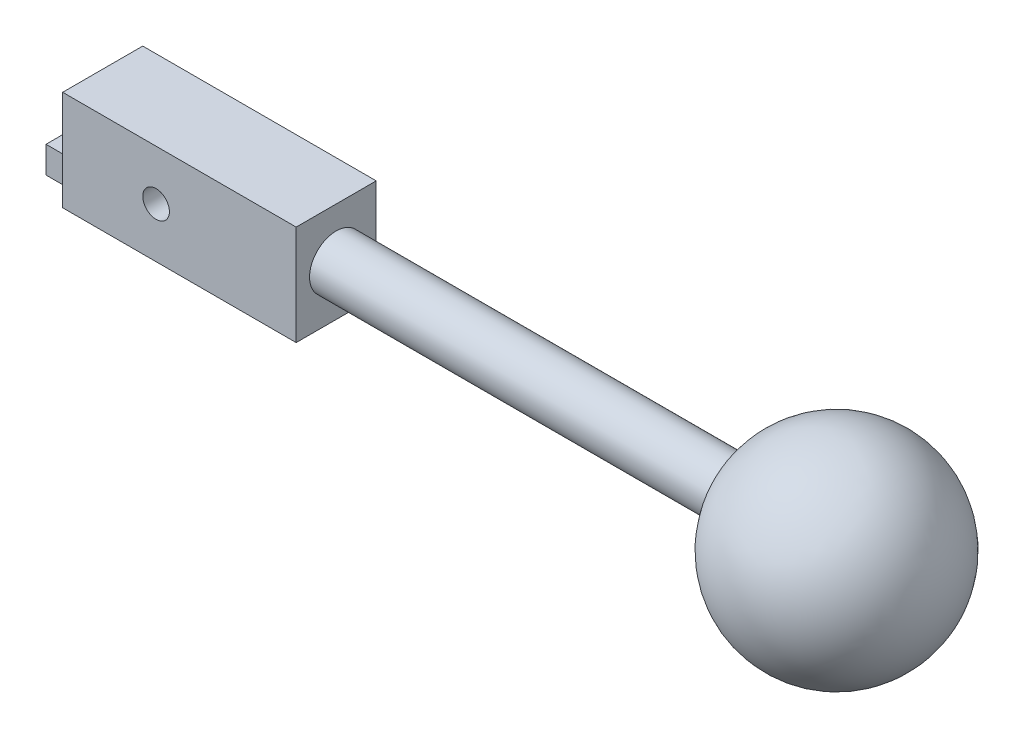
ISO-10303-21;
HEADER;
FILE_DESCRIPTION(('STEP AP214'),'2;1');
FILE_NAME('part.step','',(''),(''),'','','');
FILE_SCHEMA(('AUTOMOTIVE_DESIGN { 1 0 10303 214 1 1 1 1 }'));
ENDSEC;
DATA;
#1=APPLICATION_CONTEXT('core data for automotive mechanical design processes');
#2=APPLICATION_PROTOCOL_DEFINITION('international standard','automotive_design',2000,#1);
#3=PRODUCT_CONTEXT('',#1,'mechanical');
#4=PRODUCT('Part','Part','',(#3));
#5=PRODUCT_RELATED_PRODUCT_CATEGORY('part','',(#4));
#6=PRODUCT_DEFINITION_FORMATION('','',#4);
#7=PRODUCT_DEFINITION_CONTEXT('part definition',#1,'design');
#8=PRODUCT_DEFINITION('design','',#6,#7);
#9=PRODUCT_DEFINITION_SHAPE('','',#8);
#10=(LENGTH_UNIT() NAMED_UNIT(*) SI_UNIT(.MILLI.,.METRE.));
#11=(NAMED_UNIT(*) PLANE_ANGLE_UNIT() SI_UNIT($,.RADIAN.));
#12=(NAMED_UNIT(*) SI_UNIT($,.STERADIAN.) SOLID_ANGLE_UNIT());
#13=UNCERTAINTY_MEASURE_WITH_UNIT(LENGTH_MEASURE(1.E-05),#10,'distance_accuracy_value','');
#14=(GEOMETRIC_REPRESENTATION_CONTEXT(3) GLOBAL_UNCERTAINTY_ASSIGNED_CONTEXT((#13)) GLOBAL_UNIT_ASSIGNED_CONTEXT((#10,
#11,#12)) REPRESENTATION_CONTEXT('',''));
#15=CARTESIAN_POINT('',(0.,0.,0.));
#16=DIRECTION('',(0.,0.,1.));
#17=DIRECTION('',(1.,0.,0.));
#18=AXIS2_PLACEMENT_3D('',#15,#16,#17);
#19=CARTESIAN_POINT('',(92.5,0.,6.));
#20=DIRECTION('',(-1.,0.,0.));
#21=DIRECTION('',(0.,0.,1.));
#22=AXIS2_PLACEMENT_3D('',#19,#20,#21);
#23=CYLINDRICAL_SURFACE('',#22,4.);
#24=CARTESIAN_POINT('',(17.5,0.,6.));
#25=DIRECTION('',(1.,0.,0.));
#26=DIRECTION('',(0.,0.,-1.));
#27=AXIS2_PLACEMENT_3D('',#24,#25,#26);
#28=CIRCLE('',#27,4.);
#29=CARTESIAN_POINT('',(17.5,0.,2.));
#30=VERTEX_POINT('',#29);
#31=EDGE_CURVE('E48',#30,#30,#28,.T.);
#32=ORIENTED_EDGE('',*,*,#31,.T.);
#33=EDGE_LOOP('',(#32));
#34=FACE_BOUND('',#33,.T.);
#35=CARTESIAN_POINT('',(78.043167705199,0.,6.));
#36=DIRECTION('',(1.,0.,0.));
#37=DIRECTION('',(0.,0.,-1.));
#38=AXIS2_PLACEMENT_3D('',#35,#36,#37);
#39=CIRCLE('',#38,4.);
#40=CARTESIAN_POINT('',(78.043167705199,0.,2.));
#41=VERTEX_POINT('',#40);
#42=EDGE_CURVE('E11',#41,#41,#39,.T.);
#43=ORIENTED_EDGE('',*,*,#42,.F.);
#44=EDGE_LOOP('',(#43));
#45=FACE_BOUND('',#44,.T.);
#46=ADVANCED_FACE('F39',(#34,#45),#23,.T.);
#47=CARTESIAN_POINT('',(-17.5,-7.5,12.));
#48=DIRECTION('',(1.,0.,0.));
#49=DIRECTION('',(0.,0.,-1.));
#50=AXIS2_PLACEMENT_3D('',#47,#48,#49);
#51=PLANE('',#50);
#52=DIRECTION('',(0.,-1.,0.));
#53=VECTOR('',#52,1.);
#54=CARTESIAN_POINT('',(-17.5,-7.5,3.));
#55=LINE('',#54,#53);
#56=CARTESIAN_POINT('',(-17.5,-3.5,3.));
#57=VERTEX_POINT('',#56);
#58=CARTESIAN_POINT('',(-17.5,-7.5,3.));
#59=VERTEX_POINT('',#58);
#60=EDGE_CURVE('E54',#57,#59,#55,.T.);
#61=ORIENTED_EDGE('',*,*,#60,.F.);
#62=DIRECTION('',(0.,0.,-1.));
#63=VECTOR('',#62,1.);
#64=CARTESIAN_POINT('',(-17.5,-3.5,3.));
#65=LINE('',#64,#63);
#66=CARTESIAN_POINT('',(-17.5,-3.5,9.));
#67=VERTEX_POINT('',#66);
#68=EDGE_CURVE('E124',#67,#57,#65,.T.);
#69=ORIENTED_EDGE('',*,*,#68,.F.);
#70=DIRECTION('',(0.,1.,0.));
#71=VECTOR('',#70,1.);
#72=CARTESIAN_POINT('',(-17.5,-7.5,9.));
#73=LINE('',#72,#71);
#74=CARTESIAN_POINT('',(-17.5,-7.5,9.));
#75=VERTEX_POINT('',#74);
#76=EDGE_CURVE('E175',#75,#67,#73,.T.);
#77=ORIENTED_EDGE('',*,*,#76,.F.);
#78=DIRECTION('',(0.,0.,-1.));
#79=VECTOR('',#78,1.);
#80=CARTESIAN_POINT('',(-17.5,-7.5,12.));
#81=LINE('',#80,#79);
#82=CARTESIAN_POINT('',(-17.5,-7.5,12.));
#83=VERTEX_POINT('',#82);
#84=EDGE_CURVE('E151',#83,#75,#81,.T.);
#85=ORIENTED_EDGE('',*,*,#84,.F.);
#86=DIRECTION('',(0.,-1.,0.));
#87=VECTOR('',#86,1.);
#88=CARTESIAN_POINT('',(-17.5,-7.5,12.));
#89=LINE('',#88,#87);
#90=CARTESIAN_POINT('',(-17.5,7.5,12.));
#91=VERTEX_POINT('',#90);
#92=EDGE_CURVE('E142',#91,#83,#89,.T.);
#93=ORIENTED_EDGE('',*,*,#92,.F.);
#94=DIRECTION('',(0.,0.,-1.));
#95=VECTOR('',#94,1.);
#96=CARTESIAN_POINT('',(-17.5,7.5,12.));
#97=LINE('',#96,#95);
#98=CARTESIAN_POINT('',(-17.5,7.5,0.));
#99=VERTEX_POINT('',#98);
#100=EDGE_CURVE('E153',#91,#99,#97,.T.);
#101=ORIENTED_EDGE('',*,*,#100,.T.);
#102=DIRECTION('',(0.,-1.,0.));
#103=VECTOR('',#102,1.);
#104=CARTESIAN_POINT('',(-17.5,-7.5,0.));
#105=LINE('',#104,#103);
#106=CARTESIAN_POINT('',(-17.5,-7.5,0.));
#107=VERTEX_POINT('',#106);
#108=EDGE_CURVE('E150',#99,#107,#105,.T.);
#109=ORIENTED_EDGE('',*,*,#108,.T.);
#110=EDGE_CURVE('E58',#59,#107,#81,.T.);
#111=ORIENTED_EDGE('',*,*,#110,.F.);
#112=EDGE_LOOP('',(#61,#69,#77,#85,#93,#101,#109,#111));
#113=FACE_BOUND('',#112,.T.);
#114=ADVANCED_FACE('F182',(#113),#51,.F.);
#115=CARTESIAN_POINT('',(17.5,-7.5,12.));
#116=DIRECTION('',(-1.,0.,0.));
#117=DIRECTION('',(0.,0.,1.));
#118=AXIS2_PLACEMENT_3D('',#115,#116,#117);
#119=PLANE('',#118);
#120=ORIENTED_EDGE('',*,*,#31,.F.);
#121=EDGE_LOOP('',(#120));
#122=FACE_BOUND('',#121,.T.);
#123=DIRECTION('',(0.,1.,0.));
#124=VECTOR('',#123,1.);
#125=CARTESIAN_POINT('',(17.5,-7.5,0.));
#126=LINE('',#125,#124);
#127=CARTESIAN_POINT('',(17.5,-7.5,0.));
#128=VERTEX_POINT('',#127);
#129=CARTESIAN_POINT('',(17.5,7.5,0.));
#130=VERTEX_POINT('',#129);
#131=EDGE_CURVE('E127',#128,#130,#126,.T.);
#132=ORIENTED_EDGE('',*,*,#131,.T.);
#133=DIRECTION('',(0.,0.,-1.));
#134=VECTOR('',#133,1.);
#135=CARTESIAN_POINT('',(17.5,7.5,12.));
#136=LINE('',#135,#134);
#137=CARTESIAN_POINT('',(17.5,7.5,12.));
#138=VERTEX_POINT('',#137);
#139=EDGE_CURVE('E160',#138,#130,#136,.T.);
#140=ORIENTED_EDGE('',*,*,#139,.F.);
#141=DIRECTION('',(0.,1.,0.));
#142=VECTOR('',#141,1.);
#143=CARTESIAN_POINT('',(17.5,-7.5,12.));
#144=LINE('',#143,#142);
#145=CARTESIAN_POINT('',(17.5,-7.5,12.));
#146=VERTEX_POINT('',#145);
#147=EDGE_CURVE('E132',#146,#138,#144,.T.);
#148=ORIENTED_EDGE('',*,*,#147,.F.);
#149=DIRECTION('',(0.,0.,-1.));
#150=VECTOR('',#149,1.);
#151=CARTESIAN_POINT('',(17.5,-7.5,12.));
#152=LINE('',#151,#150);
#153=EDGE_CURVE('E144',#146,#128,#152,.T.);
#154=ORIENTED_EDGE('',*,*,#153,.T.);
#155=EDGE_LOOP('',(#132,#140,#148,#154));
#156=FACE_BOUND('',#155,.T.);
#157=ADVANCED_FACE('F41',(#122,#156),#119,.F.);
#158=CARTESIAN_POINT('',(-17.5,7.5,12.));
#159=DIRECTION('',(0.,-1.,0.));
#160=DIRECTION('',(0.,0.,-1.));
#161=AXIS2_PLACEMENT_3D('',#158,#159,#160);
#162=PLANE('',#161);
#163=DIRECTION('',(-1.,0.,0.));
#164=VECTOR('',#163,1.);
#165=CARTESIAN_POINT('',(-17.5,7.5,0.));
#166=LINE('',#165,#164);
#167=EDGE_CURVE('E126',#130,#99,#166,.T.);
#168=ORIENTED_EDGE('',*,*,#167,.T.);
#169=ORIENTED_EDGE('',*,*,#100,.F.);
#170=DIRECTION('',(-1.,0.,0.));
#171=VECTOR('',#170,1.);
#172=CARTESIAN_POINT('',(-17.5,7.5,12.));
#173=LINE('',#172,#171);
#174=EDGE_CURVE('E138',#138,#91,#173,.T.);
#175=ORIENTED_EDGE('',*,*,#174,.F.);
#176=ORIENTED_EDGE('',*,*,#139,.T.);
#177=EDGE_LOOP('',(#168,#169,#175,#176));
#178=FACE_BOUND('',#177,.T.);
#179=ADVANCED_FACE('F200',(#178),#162,.F.);
#180=CARTESIAN_POINT('',(-17.5,-7.5,12.));
#181=DIRECTION('',(0.,1.,0.));
#182=DIRECTION('',(0.,0.,1.));
#183=AXIS2_PLACEMENT_3D('',#180,#181,#182);
#184=PLANE('',#183);
#185=DIRECTION('',(1.,0.,0.));
#186=VECTOR('',#185,1.);
#187=CARTESIAN_POINT('',(-17.5,-7.5,0.));
#188=LINE('',#187,#186);
#189=EDGE_CURVE('E139',#107,#128,#188,.T.);
#190=ORIENTED_EDGE('',*,*,#189,.T.);
#191=ORIENTED_EDGE('',*,*,#153,.F.);
#192=DIRECTION('',(1.,0.,0.));
#193=VECTOR('',#192,1.);
#194=CARTESIAN_POINT('',(-17.5,-7.5,12.));
#195=LINE('',#194,#193);
#196=EDGE_CURVE('E141',#83,#146,#195,.T.);
#197=ORIENTED_EDGE('',*,*,#196,.F.);
#198=ORIENTED_EDGE('',*,*,#84,.T.);
#199=DIRECTION('',(1.,0.,0.));
#200=VECTOR('',#199,1.);
#201=CARTESIAN_POINT('',(-23.,-7.5,9.));
#202=LINE('',#201,#200);
#203=CARTESIAN_POINT('',(-23.,-7.5,9.));
#204=VERTEX_POINT('',#203);
#205=EDGE_CURVE('E109',#204,#75,#202,.T.);
#206=ORIENTED_EDGE('',*,*,#205,.F.);
#207=DIRECTION('',(0.,0.,1.));
#208=VECTOR('',#207,1.);
#209=CARTESIAN_POINT('',(-23.,-7.5,3.));
#210=LINE('',#209,#208);
#211=CARTESIAN_POINT('',(-23.,-7.5,3.));
#212=VERTEX_POINT('',#211);
#213=EDGE_CURVE('E101',#212,#204,#210,.T.);
#214=ORIENTED_EDGE('',*,*,#213,.F.);
#215=DIRECTION('',(1.,0.,0.));
#216=VECTOR('',#215,1.);
#217=CARTESIAN_POINT('',(-23.,-7.5,3.));
#218=LINE('',#217,#216);
#219=EDGE_CURVE('E110',#212,#59,#218,.T.);
#220=ORIENTED_EDGE('',*,*,#219,.T.);
#221=ORIENTED_EDGE('',*,*,#110,.T.);
#222=EDGE_LOOP('',(#190,#191,#197,#198,#206,#214,#220,#221));
#223=FACE_BOUND('',#222,.T.);
#224=ADVANCED_FACE('F102',(#223),#184,.F.);
#225=CARTESIAN_POINT('',(0.,0.,12.));
#226=DIRECTION('',(0.,0.,-1.));
#227=DIRECTION('',(-1.,0.,0.));
#228=AXIS2_PLACEMENT_3D('',#225,#226,#227);
#229=PLANE('',#228);
#230=CARTESIAN_POINT('',(-3.5,0.,12.));
#231=DIRECTION('',(0.,0.,1.));
#232=DIRECTION('',(1.,0.,0.));
#233=AXIS2_PLACEMENT_3D('',#230,#231,#232);
#234=CIRCLE('',#233,2.);
#235=CARTESIAN_POINT('',(-1.5,0.,12.));
#236=VERTEX_POINT('',#235);
#237=EDGE_CURVE('E168',#236,#236,#234,.T.);
#238=ORIENTED_EDGE('',*,*,#237,.F.);
#239=EDGE_LOOP('',(#238));
#240=FACE_BOUND('',#239,.T.);
#241=ORIENTED_EDGE('',*,*,#147,.T.);
#242=ORIENTED_EDGE('',*,*,#174,.T.);
#243=ORIENTED_EDGE('',*,*,#92,.T.);
#244=ORIENTED_EDGE('',*,*,#196,.T.);
#245=EDGE_LOOP('',(#241,#242,#243,#244));
#246=FACE_BOUND('',#245,.T.);
#247=ADVANCED_FACE('F186',(#240,#246),#229,.F.);
#248=CARTESIAN_POINT('',(0.,0.,0.));
#249=DIRECTION('',(0.,0.,-1.));
#250=DIRECTION('',(-1.,0.,0.));
#251=AXIS2_PLACEMENT_3D('',#248,#249,#250);
#252=PLANE('',#251);
#253=CARTESIAN_POINT('',(-3.5,0.,0.));
#254=DIRECTION('',(0.,0.,-1.));
#255=DIRECTION('',(-1.,0.,0.));
#256=AXIS2_PLACEMENT_3D('',#253,#254,#255);
#257=CIRCLE('',#256,2.);
#258=CARTESIAN_POINT('',(-5.5,0.,0.));
#259=VERTEX_POINT('',#258);
#260=EDGE_CURVE('E43',#259,#259,#257,.T.);
#261=ORIENTED_EDGE('',*,*,#260,.F.);
#262=EDGE_LOOP('',(#261));
#263=FACE_BOUND('',#262,.T.);
#264=ORIENTED_EDGE('',*,*,#131,.F.);
#265=ORIENTED_EDGE('',*,*,#189,.F.);
#266=ORIENTED_EDGE('',*,*,#108,.F.);
#267=ORIENTED_EDGE('',*,*,#167,.F.);
#268=EDGE_LOOP('',(#264,#265,#266,#267));
#269=FACE_BOUND('',#268,.T.);
#270=ADVANCED_FACE('F193',(#263,#269),#252,.T.);
#271=CARTESIAN_POINT('',(-23.,-7.5,3.));
#272=DIRECTION('',(0.,0.,1.));
#273=DIRECTION('',(1.,0.,0.));
#274=AXIS2_PLACEMENT_3D('',#271,#272,#273);
#275=PLANE('',#274);
#276=ORIENTED_EDGE('',*,*,#60,.T.);
#277=ORIENTED_EDGE('',*,*,#219,.F.);
#278=DIRECTION('',(0.,-1.,0.));
#279=VECTOR('',#278,1.);
#280=CARTESIAN_POINT('',(-23.,-7.5,3.));
#281=LINE('',#280,#279);
#282=CARTESIAN_POINT('',(-23.,-3.5,3.));
#283=VERTEX_POINT('',#282);
#284=EDGE_CURVE('E112',#283,#212,#281,.T.);
#285=ORIENTED_EDGE('',*,*,#284,.F.);
#286=DIRECTION('',(1.,0.,0.));
#287=VECTOR('',#286,1.);
#288=CARTESIAN_POINT('',(-23.,-3.5,3.));
#289=LINE('',#288,#287);
#290=EDGE_CURVE('E167',#283,#57,#289,.T.);
#291=ORIENTED_EDGE('',*,*,#290,.T.);
#292=EDGE_LOOP('',(#276,#277,#285,#291));
#293=FACE_BOUND('',#292,.T.);
#294=ADVANCED_FACE('F123',(#293),#275,.F.);
#295=CARTESIAN_POINT('',(-23.,-7.5,9.));
#296=DIRECTION('',(0.,0.,-1.));
#297=DIRECTION('',(-1.,0.,0.));
#298=AXIS2_PLACEMENT_3D('',#295,#296,#297);
#299=PLANE('',#298);
#300=ORIENTED_EDGE('',*,*,#76,.T.);
#301=DIRECTION('',(1.,0.,0.));
#302=VECTOR('',#301,1.);
#303=CARTESIAN_POINT('',(-23.,-3.5,9.));
#304=LINE('',#303,#302);
#305=CARTESIAN_POINT('',(-23.,-3.5,9.));
#306=VERTEX_POINT('',#305);
#307=EDGE_CURVE('E134',#306,#67,#304,.T.);
#308=ORIENTED_EDGE('',*,*,#307,.F.);
#309=DIRECTION('',(0.,1.,0.));
#310=VECTOR('',#309,1.);
#311=CARTESIAN_POINT('',(-23.,-7.5,9.));
#312=LINE('',#311,#310);
#313=EDGE_CURVE('E113',#204,#306,#312,.T.);
#314=ORIENTED_EDGE('',*,*,#313,.F.);
#315=ORIENTED_EDGE('',*,*,#205,.T.);
#316=EDGE_LOOP('',(#300,#308,#314,#315));
#317=FACE_BOUND('',#316,.T.);
#318=ADVANCED_FACE('F181',(#317),#299,.F.);
#319=CARTESIAN_POINT('',(-23.,-3.5,3.));
#320=DIRECTION('',(0.,-1.,0.));
#321=DIRECTION('',(0.,0.,-1.));
#322=AXIS2_PLACEMENT_3D('',#319,#320,#321);
#323=PLANE('',#322);
#324=ORIENTED_EDGE('',*,*,#68,.T.);
#325=ORIENTED_EDGE('',*,*,#290,.F.);
#326=DIRECTION('',(0.,0.,-1.));
#327=VECTOR('',#326,1.);
#328=CARTESIAN_POINT('',(-23.,-3.5,3.));
#329=LINE('',#328,#327);
#330=EDGE_CURVE('E118',#306,#283,#329,.T.);
#331=ORIENTED_EDGE('',*,*,#330,.F.);
#332=ORIENTED_EDGE('',*,*,#307,.T.);
#333=EDGE_LOOP('',(#324,#325,#331,#332));
#334=FACE_BOUND('',#333,.T.);
#335=ADVANCED_FACE('F177',(#334),#323,.F.);
#336=CARTESIAN_POINT('',(-23.,0.,0.));
#337=DIRECTION('',(1.,0.,0.));
#338=DIRECTION('',(0.,0.,-1.));
#339=AXIS2_PLACEMENT_3D('',#336,#337,#338);
#340=PLANE('',#339);
#341=ORIENTED_EDGE('',*,*,#284,.T.);
#342=ORIENTED_EDGE('',*,*,#213,.T.);
#343=ORIENTED_EDGE('',*,*,#313,.T.);
#344=ORIENTED_EDGE('',*,*,#330,.T.);
#345=EDGE_LOOP('',(#341,#342,#343,#344));
#346=FACE_BOUND('',#345,.T.);
#347=ADVANCED_FACE('F120',(#346),#340,.F.);
#348=CARTESIAN_POINT('',(92.5,0.,6.));
#349=DIRECTION('',(0.,0.,-1.));
#350=DIRECTION('',(1.,0.,0.));
#351=AXIS2_PLACEMENT_3D('',#348,#349,#350);
#352=SPHERICAL_SURFACE('',#351,15.);
#353=CARTESIAN_POINT('',(92.5,0.,6.));
#354=DIRECTION('',(1.,0.,0.));
#355=DIRECTION('',(0.,0.,-1.));
#356=AXIS2_PLACEMENT_3D('',#353,#354,#355);
#357=SPHERICAL_SURFACE('',#356,15.);
#358=ORIENTED_EDGE('',*,*,#42,.T.);
#359=EDGE_LOOP('',(#358));
#360=FACE_BOUND('',#359,.T.);
#361=ADVANCED_FACE('F211',(#360),#357,.T.);
#362=CARTESIAN_POINT('',(-3.5,0.,-63.));
#363=DIRECTION('',(0.,0.,1.));
#364=DIRECTION('',(1.,0.,0.));
#365=AXIS2_PLACEMENT_3D('',#362,#363,#364);
#366=CYLINDRICAL_SURFACE('',#365,2.);
#367=ORIENTED_EDGE('',*,*,#260,.T.);
#368=EDGE_LOOP('',(#367));
#369=FACE_BOUND('',#368,.T.);
#370=ORIENTED_EDGE('',*,*,#237,.T.);
#371=EDGE_LOOP('',(#370));
#372=FACE_BOUND('',#371,.T.);
#373=ADVANCED_FACE('F268',(#369,#372),#366,.F.);
#374=CLOSED_SHELL('',(#46,#114,#157,#179,#224,#247,#270,#294,#318,#335,#347,#361,#373));
#375=MANIFOLD_SOLID_BREP('B2',#374);
#376=ADVANCED_BREP_SHAPE_REPRESENTATION('',(#18,#375),#14);
#377=SHAPE_DEFINITION_REPRESENTATION(#9,#376);
ENDSEC;
END-ISO-10303-21;
